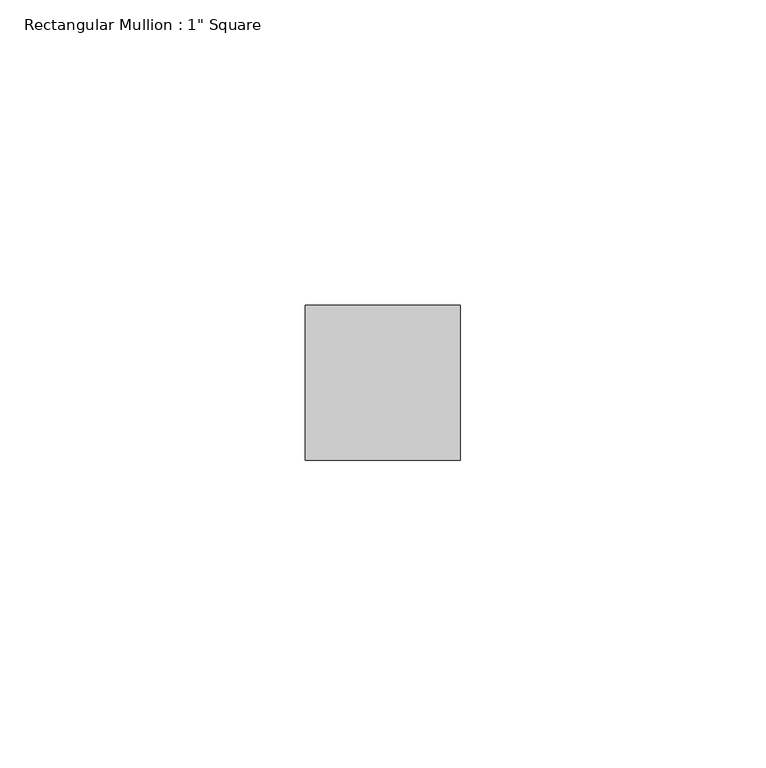
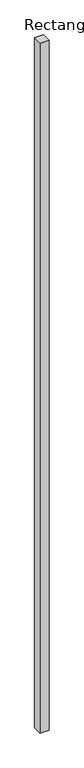
"""IFC4 building model written with IfcOpenShell, lengths in millimetres: member geometry."""

from ifc_helpers import new_model, si_unit, frame, origin, place, context, project, spatial, polyline, outline, extrude, source, transform, mapped, element, save


def member_0682bd88(model_context):
    return source(origin(), model_context, "Body", "SweptSolid", [
        extrude(outline(polyline([(0.0, 12.7), (0.0, -12.7), (-25.4, -12.7), (-25.4, 12.7), (0.0, 12.7)])), frame((0.0, 0.0, -2060.8644013), z_axis=(0.0, 0.0, 1.0), x_axis=(1.0, 0.0, 0.0)), (0.0, 0.0, 1.0), 2060.8644013),
    ])


if __name__ == "__main__":
    model = new_model("IFC4")
    model_context = context("Model", 3, world=origin())
    ifc_project = project(units=[si_unit("LENGTHUNIT", "METRE", prefix="MILLI")], contexts=[model_context])
    site = spatial("IfcSite", under=ifc_project)
    building = spatial("IfcBuilding", under=site)
    placement = place(None, origin())
    member_shape = member_0682bd88(model_context)
    element("IfcMember", 1, ObjectType="Rectangular Mullion : 1\" Square", at=placement, inside=building, context=model_context, shape_type="MappedRepresentation", body=[
        mapped(member_shape, transform((0.0, 0.0, 0.0), x_axis=(1.0, 0.0, 0.0), y_axis=(0.0, 1.0, 0.0), z_axis=(0.0, 0.0, 1.0))),
    ])
    save(model, "model.ifc")

# Revit data of these elements
# Type "Rectangular Mullion : 1\" Square"
#   built-in parameter 1007304 = 0.0833333 (stored number, unit not read)
#   built-in parameter 1007301 = 0.0416667 (stored number, unit not read)
#   built-in parameter 1007300 = 0.0416667 (stored number, unit not read)
